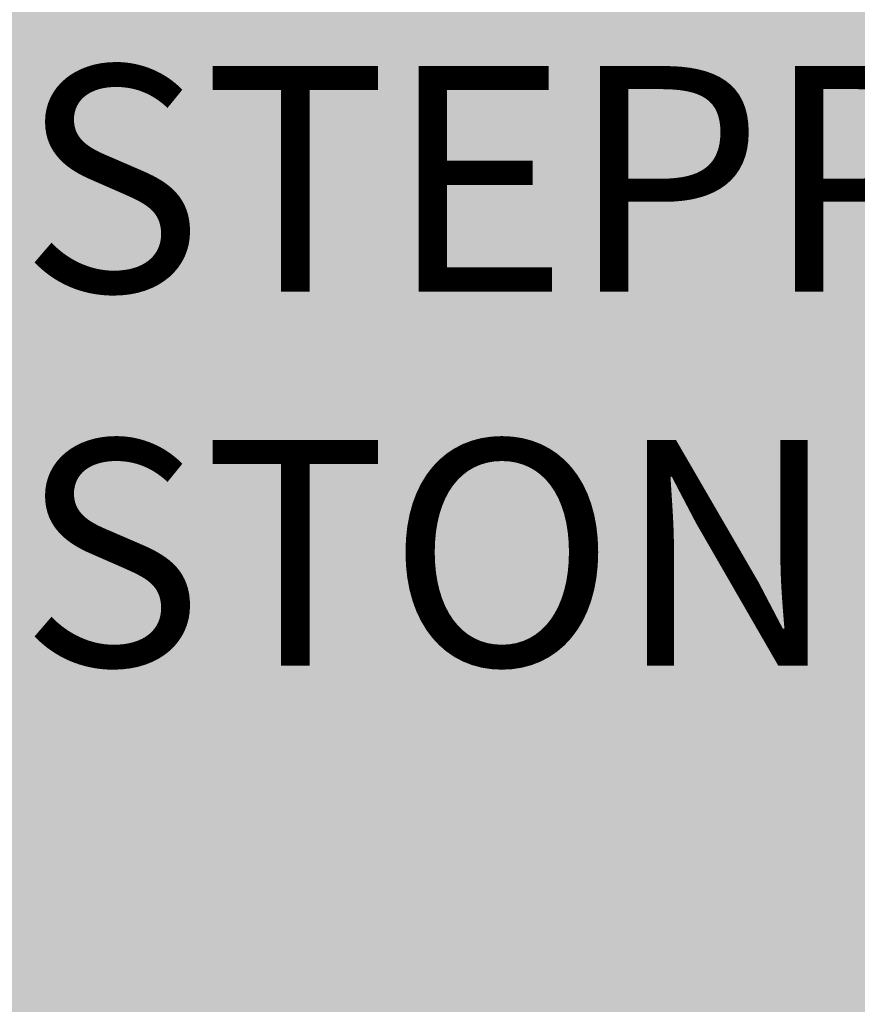
# Model space of a CAD drawing. Units: inches. Extents: x 1704 to 6393, y -157 to 1172.
# Tile 66 of 122: x 1937 to 1987, y 920 to 980. Entities that reach past the tile are written whole.
import ezdxf

# ---------------------------------------------------------------- set-up
doc = ezdxf.new("R2010")
doc.units = ezdxf.units.IN
doc.header["$MEASUREMENT"] = 0
doc.layers.add('A-ANNO-DIMS', color=7, linetype='Continuous', lineweight=13)
doc.layers.add('A-AREA-IDEN', color=7, linetype='Continuous', lineweight=18)
doc.layers.add('L-HRDS-PATT', color=9, linetype='Continuous', lineweight=13, true_color=0xc5c1ba)
doc.styles.get("Standard").update_dxf_attribs({"font": 'arial.ttf'})
doc.dimstyles.get("Standard").update_dxf_attribs({"dimtxt": 6, "dimasz": 2, "dimexe": 0.18, "dimexo": 0.0625, "dimgap": 0.09, "dimtad": 0, "dimtih": 1, "dimtoh": 1, "dimdec": 1, "dimzin": 0, "dimdsep": 46, "dimlunit": 3, "dimtxsty": 'Standard', "dimblk": 'ARCHTICK', "dimcen": 0.09, "dimadec": 0, "dimazin": 0, "dimtfac": 1, "dimtdec": 1, "dimtofl": 0, "dimtmove": 0, "dimatfit": 3, "dimfxl": 1, "dimtolj": 1, "dimtzin": 0, "dimarcsym": 0})

# ---------------------------------------------------------------- blocks, each defined once
blk = doc.blocks.new('_ArchTick')
at = {"color": 0, "linetype": 'ByBlock', "const_width": 0.15}
blk.add_lwpolyline([(-0.5, -0.5), (0.5, 0.5)], dxfattribs=at)
blk = doc.blocks.new('*D94')
at = {"layer": 'A-ANNO-DIMS', "color": 0, "lineweight": -2, "transparency": 16777216}
for p, q in [((1898.349, 895.275), (1898.349, 1105.287)), ((1898.349, 1105.107), (1979.39, 1105.107)), ((2073.349, 1105.107), (1992.307, 1105.107)), ((2073.349, 895.275), (2073.349, 1105.287))]:
    blk.add_line(p, q, dxfattribs=at)
at = {"layer": 'Defpoints', "color": 0, "lineweight": -3, "transparency": 16777216}
for p in [(2073.349, 1105.107), (1898.349, 895.213), (2073.349, 895.213)]:
    blk.add_point(p, dxfattribs=at)
at = {"layer": 'A-ANNO-DIMS', "color": 0, "lineweight": -2, "transparency": 16777216, "xscale": 2, "yscale": 2, "zscale": 2, "rotation": 180}
blk.add_blockref('_ArchTick', (1898.349, 1105.107), dxfattribs=at)
at = {"layer": 'A-ANNO-DIMS', "color": 0, "lineweight": -2, "transparency": 16777216, "xscale": 2, "yscale": 2, "zscale": 2}
blk.add_blockref('_ArchTick', (2073.349, 1105.107), dxfattribs=at)
at = {"layer": 'A-ANNO-DIMS', "color": 0, "transparency": 16777216, "insert": (1985.849, 1105.107), "char_height": 6, "attachment_point": 5}
blk.add_mtext('\\A1;175', dxfattribs=at)

msp = doc.modelspace()

# ---------------------------------------------------------------- hatches: boundary and pattern name
at = {"layer": 'L-HRDS-PATT', "transparency": 33554643}
h = msp.add_hatch(color=256, dxfattribs=at)
h.dxf.hatch_style = 1
h.paths.add_polyline_path([(2065.589, 1033.213), (1898.349, 1033.213), (1898.349, 895.213), (2065.589, 895.213)])

# ---------------------------------------------------------------- texts
at = {"layer": 'A-AREA-IDEN'}
for s, p in [('STEPPING', (1936.64, 963.579)), ('STONE', (1936.64, 940.915))]:
    msp.add_text(s, height=13.6672, dxfattribs=at).set_placement(p)

# ---------------------------------------------------------------- dimensions: what is measured, and where the dimension line sits
at = {"layer": 'A-ANNO-DIMS'}
dim = msp.add_linear_dim(base=(2073.349, 1105.107), p1=(1898.349, 895.213), p2=(2073.349, 895.213), dimstyle='Standard', override={"dimdec": 0, "dimlfac": 1, "dimrnd": 0, "dimzin": 0, "dimdsep": 46, "dimlunit": 2}, dxfattribs=at)
dim.commit()
dim.dimension.update_dxf_attribs({"geometry": '*D94', "text_midpoint": (1985.849, 1105.107)})

doc.saveas('drawing.dxf')
